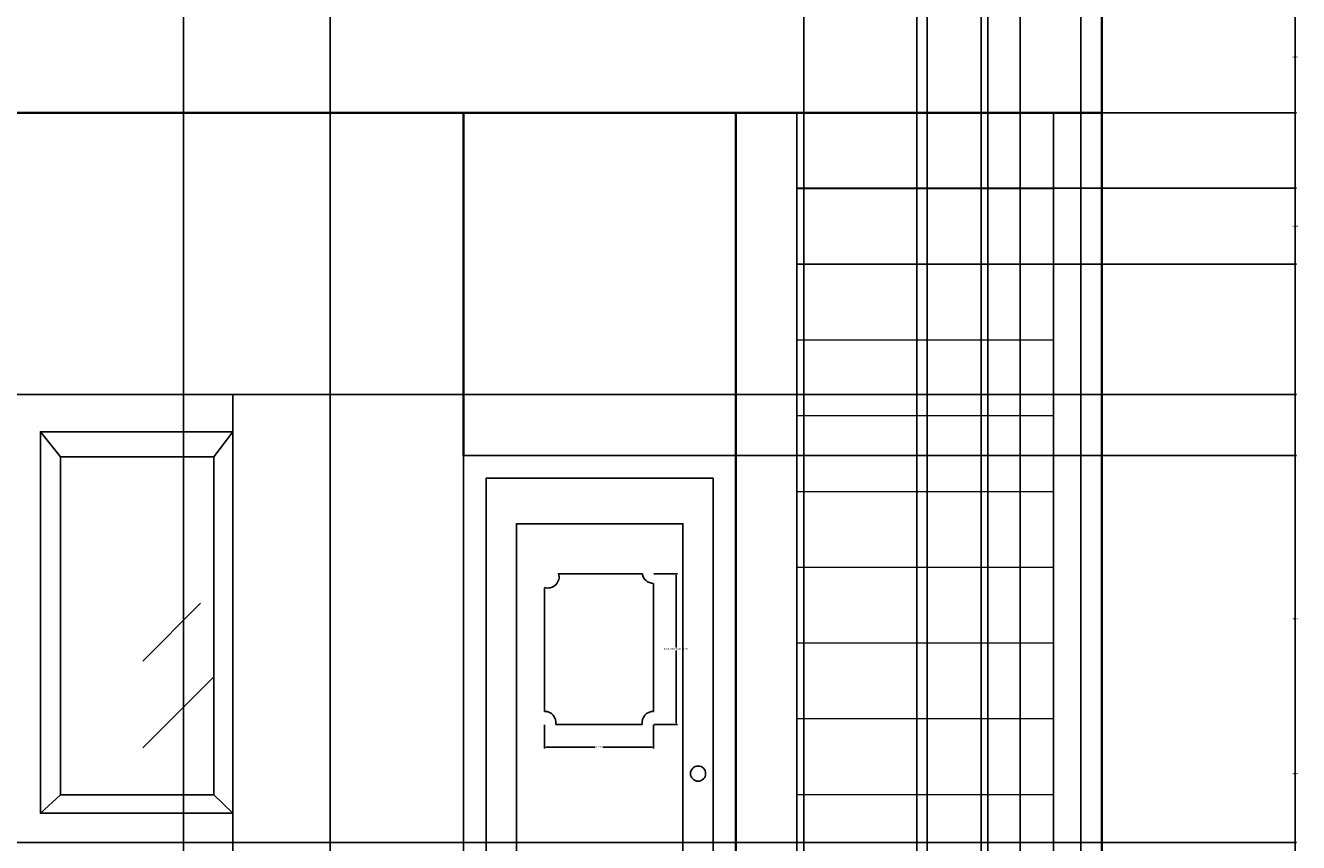
# Model space of a CAD drawing. Units: inches. Extents: x 93 to 565, y 123 to 656.
# Tile 4 of 18: x 397 to 565, y 217 to 324. Entities that reach past the tile are written whole.
import ezdxf

# ---------------------------------------------------------------- set-up
doc = ezdxf.new("R2010")
doc.units = ezdxf.units.IN
doc.header["$MEASUREMENT"] = 0
for name, color, linetype, lineweight in [('A-ANNO-DIMS', 2, 'Continuous', 18), ('A-DOOR', 3, 'Continuous', 25), ('A-ELEV', 7, 'Continuous', 35), ('A-FLOR-STRS', 6, 'Continuous', 18), ('A-GLAZ', 4, 'Continuous', 25)]:
    doc.layers.add(name, color=color, linetype=linetype, lineweight=lineweight)
doc.styles.get("Standard").update_dxf_attribs({"font": 'arial.ttf'})
doc.dimstyles.get("Standard").update_dxf_attribs({"dimtxt": 0.18, "dimasz": 0.18, "dimexe": 0.18, "dimexo": 0.0625, "dimgap": 0.09, "dimtad": 0, "dimtih": 1, "dimtoh": 1, "dimdec": 4, "dimzin": 0, "dimdsep": 46, "dimtxsty": 'Standard', "dimcen": 0.09, "dimadec": 0, "dimazin": 0, "dimtfac": 1, "dimtdec": 4, "dimtofl": 0, "dimtmove": 0, "dimatfit": 3, "dimfxl": 1, "dimtolj": 1, "dimtzin": 0, "dimarcsym": 0})

# ---------------------------------------------------------------- blocks, each defined once
blk = doc.blocks.new('*U4')
blk.add_lwpolyline([(3.12, 0.01), (0.12, 0.01), (0.12, 84.01), (36.12, 84.01), (36.12, 0.01), (33.12, 0.01)])
for points in [[(33.12, 80.99), (33.12, 0.01), (3.12, 0.01), (3.12, 80.99)], [(29.12, 6.01), (29.12, 74.99), (7.12, 74.99), (7.12, 6.01)]]:
    blk.add_lwpolyline(points, close=True)
blk.add_circle((31.12, 42.01), 1)
blk = doc.blocks.new('DOOR-PANEL-UPPER')
for points in [[(1.85, 19.9), (12.89, 19.9)], [(14.37, 18.62), (14.37, 1.72)], [(0, 1.72), (0, 18.05)], [(12.89, 0), (1.48, 0)]]:
    blk.add_lwpolyline(points)
for centre, start, end in [((0.41, 19.5), 254.1895, 15.8285), ((14.37, 20.12), 188.4141, 270), ((0, 0.22), 351.5859, 90), ((14.37, 0.22), 90, 188.4141)]:
    blk.add_arc(centre, 1.5, start, end)
blk = doc.blocks.new('WIN-CASEMENT-LARGE')
blk.add_lwpolyline([(2.67, 44.6), (0, 47.91), (25.42, 47.91), (22.89, 44.6)])
blk.add_lwpolyline([(2.67, 44.6), (22.89, 44.6), (22.89, 0), (2.67, 0)], close=True)
blk = doc.blocks.new('*D22')
at = {"layer": 'A-ANNO-DIMS', "color": 0, "lineweight": -2, "transparency": 16777216}
for p, q in [((479.94, 252.12), (483.04, 252.12)), ((482.86, 251.94), (482.86, 242.36)), ((482.86, 232.4), (482.86, 241.99)), ((479.94, 232.22), (483.04, 232.22))]:
    blk.add_line(p, q, dxfattribs=at)
at = {"layer": 'A-ANNO-DIMS', "color": 0, "transparency": 16777216}
for points in [[(482.83, 251.94), (482.89, 251.94), (482.86, 252.12)], [(482.83, 232.4), (482.89, 232.4), (482.86, 232.22)]]:
    blk.add_solid(points, dxfattribs=at)
at = {"layer": 'Defpoints', "color": 0, "transparency": 16777216}
for p in [(479.88, 252.12), (482.86, 252.12), (479.88, 232.22)]:
    blk.add_point(p, dxfattribs=at)
at = {"layer": 'A-ANNO-DIMS', "color": 0, "transparency": 16777216, "insert": (482.86, 242.17), "char_height": 0.18, "attachment_point": 5}
blk.add_mtext('\\A1;DOOR UPPER PANEL 20 TYP.', dxfattribs=at)
blk = doc.blocks.new('*D23')
at = {"layer": 'A-ANNO-DIMS', "color": 0, "lineweight": -2, "transparency": 16777216}
for p, q in [((465.5, 232.16), (465.5, 229.05)), ((479.88, 232.16), (479.88, 229.05)), ((465.68, 229.23), (472.17, 229.23)), ((479.7, 229.23), (473.21, 229.23))]:
    blk.add_line(p, q, dxfattribs=at)
at = {"layer": 'A-ANNO-DIMS', "color": 0, "transparency": 16777216}
for points in [[(465.68, 229.26), (465.68, 229.2), (465.5, 229.23)], [(479.7, 229.26), (479.7, 229.2), (479.88, 229.23)]]:
    blk.add_solid(points, dxfattribs=at)
at = {"layer": 'Defpoints', "color": 0, "transparency": 16777216}
for p in [(465.5, 232.22), (479.88, 232.22), (479.88, 229.23)]:
    blk.add_point(p, dxfattribs=at)
at = {"layer": 'A-ANNO-DIMS', "color": 0, "transparency": 16777216, "insert": (472.69, 229.23), "char_height": 0.18, "attachment_point": 5}
blk.add_mtext('\\A1;14 TYP.', dxfattribs=at)
blk = doc.blocks.new('*D29')
at = {"layer": 'A-ANNO-DIMS', "color": 0, "lineweight": -2, "transparency": 16777216}
for p, q in [((437.19, 594.34), (437.19, 134)), ((295.69, 183.67), (295.69, 134)), ((295.87, 134.18), (366.05, 134.18)), ((437.01, 134.18), (366.82, 134.18))]:
    blk.add_line(p, q, dxfattribs=at)
at = {"layer": 'A-ANNO-DIMS', "color": 0, "transparency": 16777216}
for points in [[(295.87, 134.21), (295.87, 134.15), (295.69, 134.18)], [(437.01, 134.21), (437.01, 134.15), (437.19, 134.18)]]:
    blk.add_solid(points, dxfattribs=at)
at = {"layer": 'Defpoints', "color": 0, "transparency": 16777216}
for p in [(437.19, 594.4), (295.69, 183.73), (437.19, 134.18)]:
    blk.add_point(p, dxfattribs=at)
at = {"layer": 'A-ANNO-DIMS', "color": 0, "transparency": 16777216, "insert": (366.44, 134.18), "char_height": 0.18, "attachment_point": 5}
blk.add_mtext('\\A1;141.5', dxfattribs=at)
blk = doc.blocks.new('*D30')
at = {"layer": 'A-ANNO-DIMS', "color": 0, "lineweight": -2, "transparency": 16777216}
for p, q in [((437.19, 594.34), (437.19, 134)), ((539.08, 159.67), (539.08, 134)), ((437.37, 134.18), (487.75, 134.18)), ((538.9, 134.18), (488.52, 134.18))]:
    blk.add_line(p, q, dxfattribs=at)
at = {"layer": 'A-ANNO-DIMS', "color": 0, "transparency": 16777216}
for points in [[(437.37, 134.21), (437.37, 134.15), (437.19, 134.18)], [(538.9, 134.21), (538.9, 134.15), (539.08, 134.18)]]:
    blk.add_solid(points, dxfattribs=at)
at = {"layer": 'Defpoints', "color": 0, "transparency": 16777216}
for p in [(437.19, 594.4), (539.08, 159.73), (539.08, 134.18)]:
    blk.add_point(p, dxfattribs=at)
at = {"layer": 'A-ANNO-DIMS', "color": 0, "transparency": 16777216, "insert": (488.13, 134.18), "char_height": 0.18, "attachment_point": 5}
blk.add_mtext('\\A1;101.9', dxfattribs=at)
blk = doc.blocks.new('*D31')
at = {"layer": 'A-ANNO-DIMS', "color": 0, "lineweight": -2, "transparency": 16777216}
for p, q in [((417.87, 630.4), (564.81, 630.4)), ((564.63, 630.22), (564.63, 395.25)), ((564.63, 159.91), (564.63, 394.89)), ((119.14, 159.73), (564.81, 159.73))]:
    blk.add_line(p, q, dxfattribs=at)
at = {"layer": 'A-ANNO-DIMS', "color": 0, "transparency": 16777216}
for points in [[(564.6, 630.22), (564.66, 630.22), (564.63, 630.4)], [(564.6, 159.91), (564.66, 159.91), (564.63, 159.73)]]:
    blk.add_solid(points, dxfattribs=at)
at = {"layer": 'Defpoints', "color": 0, "transparency": 16777216}
for p in [(417.81, 630.4), (564.63, 630.4), (119.08, 159.73)]:
    blk.add_point(p, dxfattribs=at)
at = {"layer": 'A-ANNO-DIMS', "color": 0, "transparency": 16777216, "insert": (564.63, 395.07), "char_height": 0.18, "attachment_point": 5}
blk.add_mtext('\\A1;470.7', dxfattribs=at)
blk = doc.blocks.new('*D37')
at = {"layer": 'A-ANNO-DIMS', "color": 0, "lineweight": -2, "transparency": 16777216}
for p, q in [((539.14, 327.73), (564.81, 327.73)), ((564.63, 327.55), (564.63, 320.52)), ((564.63, 313.13), (564.63, 320.16)), ((539.14, 312.95), (564.81, 312.95))]:
    blk.add_line(p, q, dxfattribs=at)
at = {"layer": 'A-ANNO-DIMS', "color": 0, "transparency": 16777216}
for points in [[(564.6, 327.55), (564.66, 327.55), (564.63, 327.73)], [(564.6, 313.13), (564.66, 313.13), (564.63, 312.95)]]:
    blk.add_solid(points, dxfattribs=at)
at = {"layer": 'Defpoints', "color": 0, "transparency": 16777216}
for p in [(539.08, 327.73), (564.63, 327.73), (539.08, 312.95)]:
    blk.add_point(p, dxfattribs=at)
at = {"layer": 'A-ANNO-DIMS', "color": 0, "transparency": 16777216, "insert": (564.63, 320.34), "char_height": 0.18, "attachment_point": 5}
blk.add_mtext('\\A1;14.783', dxfattribs=at)
blk = doc.blocks.new('*D56')
at = {"layer": 'A-ANNO-DIMS', "color": 0, "lineweight": -2, "transparency": 16777216}
for p, q in [((309.74, 275.71), (309.74, 134)), ((424.3, 275.71), (424.3, 134)), ((309.92, 134.18), (366.57, 134.18)), ((424.12, 134.18), (367.48, 134.18))]:
    blk.add_line(p, q, dxfattribs=at)
at = {"layer": 'A-ANNO-DIMS', "color": 0, "transparency": 16777216}
for points in [[(309.92, 134.21), (309.92, 134.15), (309.74, 134.18)], [(424.12, 134.21), (424.12, 134.15), (424.3, 134.18)]]:
    blk.add_solid(points, dxfattribs=at)
at = {"layer": 'Defpoints', "color": 0, "transparency": 16777216}
for p in [(309.74, 275.77), (424.3, 275.77), (424.3, 134.18)]:
    blk.add_point(p, dxfattribs=at)
at = {"layer": 'A-ANNO-DIMS', "color": 0, "transparency": 16777216, "insert": (367.02, 134.18), "char_height": 0.18, "attachment_point": 5}
blk.add_mtext('\\A1;114.56', dxfattribs=at)
blk = doc.blocks.new('*D57')
at = {"layer": 'A-ANNO-DIMS', "color": 0, "lineweight": -2, "transparency": 16777216}
for p, q in [((424.37, 275.77), (564.81, 275.77)), ((564.63, 275.59), (564.63, 246.38)), ((564.63, 216.81), (564.63, 246.02)), ((424.37, 216.63), (564.81, 216.63))]:
    blk.add_line(p, q, dxfattribs=at)
at = {"layer": 'A-ANNO-DIMS', "color": 0, "transparency": 16777216}
for points in [[(564.6, 275.59), (564.66, 275.59), (564.63, 275.77)], [(564.6, 216.81), (564.66, 216.81), (564.63, 216.63)]]:
    blk.add_solid(points, dxfattribs=at)
at = {"layer": 'Defpoints', "color": 0, "transparency": 16777216}
for p in [(424.3, 275.77), (564.63, 275.77), (424.3, 216.63)]:
    blk.add_point(p, dxfattribs=at)
at = {"layer": 'A-ANNO-DIMS', "color": 0, "transparency": 16777216, "insert": (564.63, 246.2), "char_height": 0.18, "attachment_point": 5}
blk.add_mtext('\\A1;59.14', dxfattribs=at)
blk = doc.blocks.new('*D59')
at = {"layer": 'A-ANNO-DIMS', "color": 0, "lineweight": -2, "transparency": 16777216}
for p, q in [((454.77, 267.67), (454.77, 134)), ((490.77, 267.67), (490.77, 134)), ((454.95, 134.18), (472.55, 134.18)), ((490.59, 134.18), (472.99, 134.18))]:
    blk.add_line(p, q, dxfattribs=at)
at = {"layer": 'A-ANNO-DIMS', "color": 0, "transparency": 16777216}
for points in [[(454.95, 134.21), (454.95, 134.15), (454.77, 134.18)], [(490.59, 134.21), (490.59, 134.15), (490.77, 134.18)]]:
    blk.add_solid(points, dxfattribs=at)
at = {"layer": 'Defpoints', "color": 0, "transparency": 16777216}
for p in [(454.77, 267.73), (490.77, 267.73), (490.77, 134.18)]:
    blk.add_point(p, dxfattribs=at)
at = {"layer": 'A-ANNO-DIMS', "color": 0, "transparency": 16777216, "insert": (472.77, 134.18), "char_height": 0.18, "attachment_point": 5}
blk.add_mtext('\\A1;36', dxfattribs=at)
blk = doc.blocks.new('*D60')
at = {"layer": 'A-ANNO-DIMS', "color": 0, "lineweight": -2, "transparency": 16777216}
for p, q in [((490.83, 267.73), (564.81, 267.73)), ((564.63, 267.55), (564.63, 225.91)), ((564.63, 183.91), (564.63, 225.55)), ((490.83, 183.73), (564.81, 183.73))]:
    blk.add_line(p, q, dxfattribs=at)
at = {"layer": 'A-ANNO-DIMS', "color": 0, "transparency": 16777216}
for points in [[(564.6, 267.55), (564.66, 267.55), (564.63, 267.73)], [(564.6, 183.91), (564.66, 183.91), (564.63, 183.73)]]:
    blk.add_solid(points, dxfattribs=at)
at = {"layer": 'Defpoints', "color": 0, "transparency": 16777216}
for p in [(490.77, 267.73), (564.63, 267.73), (490.77, 183.73)]:
    blk.add_point(p, dxfattribs=at)
at = {"layer": 'A-ANNO-DIMS', "color": 0, "transparency": 16777216, "insert": (564.63, 225.73), "char_height": 0.18, "attachment_point": 5}
blk.add_mtext('\\A1;84', dxfattribs=at)
blk = doc.blocks.new('*D62')
at = {"layer": 'A-ANNO-DIMS', "color": 0, "lineweight": -2, "transparency": 16777216}
for p, q in [((498.79, 312.92), (498.79, 134)), ((532.69, 312.92), (532.69, 134)), ((498.97, 134.18), (515.42, 134.18)), ((532.51, 134.18), (516.07, 134.18))]:
    blk.add_line(p, q, dxfattribs=at)
at = {"layer": 'A-ANNO-DIMS', "color": 0, "transparency": 16777216}
for points in [[(498.97, 134.21), (498.97, 134.15), (498.79, 134.18)], [(532.51, 134.21), (532.51, 134.15), (532.69, 134.18)]]:
    blk.add_solid(points, dxfattribs=at)
at = {"layer": 'Defpoints', "color": 0, "transparency": 16777216}
for p in [(498.79, 312.99), (532.69, 312.99), (532.69, 134.18)]:
    blk.add_point(p, dxfattribs=at)
at = {"layer": 'A-ANNO-DIMS', "color": 0, "transparency": 16777216, "insert": (515.74, 134.18), "char_height": 0.18, "attachment_point": 5}
blk.add_mtext('\\A1;33.9', dxfattribs=at)
blk = doc.blocks.new('*D63')
at = {"layer": 'A-ANNO-DIMS', "color": 0, "lineweight": -2, "transparency": 16777216}
for p, q in [((498.86, 302.99), (564.81, 302.99)), ((564.63, 302.81), (564.63, 298.17)), ((564.63, 293.17), (564.63, 297.8)), ((498.86, 292.99), (564.81, 292.99))]:
    blk.add_line(p, q, dxfattribs=at)
at = {"layer": 'A-ANNO-DIMS', "color": 0, "transparency": 16777216}
for points in [[(564.6, 302.81), (564.66, 302.81), (564.63, 302.99)], [(564.6, 293.17), (564.66, 293.17), (564.63, 292.99)]]:
    blk.add_solid(points, dxfattribs=at)
at = {"layer": 'Defpoints', "color": 0, "transparency": 16777216}
for p in [(498.79, 302.99), (498.79, 292.99), (564.63, 292.99)]:
    blk.add_point(p, dxfattribs=at)
at = {"layer": 'A-ANNO-DIMS', "color": 0, "transparency": 16777216, "insert": (564.63, 297.99), "char_height": 0.18, "attachment_point": 5}
blk.add_mtext('\\A1;10', dxfattribs=at)
blk = doc.blocks.new('*D90')
at = {"layer": 'A-ANNO-DIMS', "color": 0, "lineweight": -2, "transparency": 16777216}
for p, q in [((417.81, 594.34), (417.81, 134)), ((437.19, 594.34), (437.19, 134)), ((417.99, 134.18), (427.11, 134.18)), ((437.01, 134.18), (427.88, 134.18))]:
    blk.add_line(p, q, dxfattribs=at)
at = {"layer": 'A-ANNO-DIMS', "color": 0, "transparency": 16777216}
for points in [[(417.99, 134.21), (417.99, 134.15), (417.81, 134.18)], [(437.01, 134.21), (437.01, 134.15), (437.19, 134.18)]]:
    blk.add_solid(points, dxfattribs=at)
at = {"layer": 'Defpoints', "color": 0, "transparency": 16777216}
for p in [(417.81, 594.4), (437.19, 594.4), (437.19, 134.18)]:
    blk.add_point(p, dxfattribs=at)
at = {"layer": 'A-ANNO-DIMS', "color": 0, "transparency": 16777216, "insert": (427.5, 134.18), "char_height": 0.18, "attachment_point": 5}
blk.add_mtext('\\A1;19.38', dxfattribs=at)
blk = doc.blocks.new('*D91')
at = {"layer": 'A-ANNO-DIMS', "color": 0, "lineweight": -2, "transparency": 16777216}
for p, q in [((499.73, 599.75), (499.73, 134)), ((437.19, 594.34), (437.19, 134)), ((437.37, 134.18), (468.07, 134.18)), ((499.55, 134.18), (468.85, 134.18))]:
    blk.add_line(p, q, dxfattribs=at)
at = {"layer": 'A-ANNO-DIMS', "color": 0, "transparency": 16777216}
for points in [[(437.37, 134.21), (437.37, 134.15), (437.19, 134.18)], [(499.55, 134.21), (499.55, 134.15), (499.73, 134.18)]]:
    blk.add_solid(points, dxfattribs=at)
at = {"layer": 'Defpoints', "color": 0, "transparency": 16777216}
for p in [(499.73, 599.82), (437.19, 594.4), (499.73, 134.18)]:
    blk.add_point(p, dxfattribs=at)
at = {"layer": 'A-ANNO-DIMS', "color": 0, "transparency": 16777216, "insert": (468.46, 134.18), "char_height": 0.18, "attachment_point": 5}
blk.add_mtext('\\A1;62.54', dxfattribs=at)
blk = doc.blocks.new('*D92')
at = {"layer": 'A-ANNO-DIMS', "color": 0, "lineweight": -2, "transparency": 16777216}
for p, q in [((523.14, 603.14), (523.14, 134)), ((499.73, 599.75), (499.73, 134)), ((499.91, 134.18), (510.97, 134.18)), ((522.96, 134.18), (511.9, 134.18))]:
    blk.add_line(p, q, dxfattribs=at)
at = {"layer": 'A-ANNO-DIMS', "color": 0, "transparency": 16777216}
for points in [[(499.91, 134.21), (499.91, 134.15), (499.73, 134.18)], [(522.96, 134.21), (522.96, 134.15), (523.14, 134.18)]]:
    blk.add_solid(points, dxfattribs=at)
at = {"layer": 'Defpoints', "color": 0, "transparency": 16777216}
for p in [(523.14, 603.2), (499.73, 599.82), (523.14, 134.18)]:
    blk.add_point(p, dxfattribs=at)
at = {"layer": 'A-ANNO-DIMS', "color": 0, "transparency": 16777216, "insert": (511.44, 134.18), "char_height": 0.18, "attachment_point": 5}
blk.add_mtext('\\A1;23.412', dxfattribs=at)
blk = doc.blocks.new('*D93')
at = {"layer": 'A-ANNO-DIMS', "color": 0, "lineweight": -2, "transparency": 16777216}
for p, q in [((523.14, 603.14), (523.14, 134)), ((539.08, 594.34), (539.08, 134)), ((523.32, 134.18), (530.66, 134.18)), ((538.9, 134.18), (531.57, 134.18))]:
    blk.add_line(p, q, dxfattribs=at)
at = {"layer": 'A-ANNO-DIMS', "color": 0, "transparency": 16777216}
for points in [[(523.32, 134.21), (523.32, 134.15), (523.14, 134.18)], [(538.9, 134.21), (538.9, 134.15), (539.08, 134.18)]]:
    blk.add_solid(points, dxfattribs=at)
at = {"layer": 'Defpoints', "color": 0, "transparency": 16777216}
for p in [(523.14, 603.2), (539.08, 594.4), (539.08, 134.18)]:
    blk.add_point(p, dxfattribs=at)
at = {"layer": 'A-ANNO-DIMS', "color": 0, "transparency": 16777216, "insert": (531.11, 134.18), "char_height": 0.18, "attachment_point": 5}
blk.add_mtext('\\A1;15.938', dxfattribs=at)
blk = doc.blocks.new('*D108')
at = {"layer": 'A-ANNO-DIMS', "color": 0, "lineweight": -2, "transparency": 16777216}
for p, q in [((437.19, 594.34), (437.19, 134)), ((295.69, 183.67), (295.69, 134)), ((295.87, 134.18), (365.93, 134.18)), ((437.01, 134.18), (366.95, 134.18))]:
    blk.add_line(p, q, dxfattribs=at)
at = {"layer": 'A-ANNO-DIMS', "color": 0, "transparency": 16777216}
for points in [[(295.87, 134.21), (295.87, 134.15), (295.69, 134.18)], [(437.01, 134.21), (437.01, 134.15), (437.19, 134.18)]]:
    blk.add_solid(points, dxfattribs=at)
at = {"layer": 'Defpoints', "color": 0, "transparency": 16777216}
for p in [(437.19, 594.4), (295.69, 183.73), (437.19, 134.18)]:
    blk.add_point(p, dxfattribs=at)
at = {"layer": 'A-ANNO-DIMS', "color": 0, "transparency": 16777216, "insert": (366.44, 134.18), "char_height": 0.18, "attachment_point": 5}
blk.add_mtext('\\A1;141.501', dxfattribs=at)
blk = doc.blocks.new('*D109')
at = {"layer": 'A-ANNO-DIMS', "color": 0, "lineweight": -2, "transparency": 16777216}
for p, q in [((437.19, 594.34), (437.19, 134)), ((539.08, 159.67), (539.08, 134)), ((437.37, 134.18), (487.63, 134.18)), ((538.9, 134.18), (488.64, 134.18))]:
    blk.add_line(p, q, dxfattribs=at)
at = {"layer": 'A-ANNO-DIMS', "color": 0, "transparency": 16777216}
for points in [[(437.37, 134.21), (437.37, 134.15), (437.19, 134.18)], [(538.9, 134.21), (538.9, 134.15), (539.08, 134.18)]]:
    blk.add_solid(points, dxfattribs=at)
at = {"layer": 'Defpoints', "color": 0, "transparency": 16777216}
for p in [(437.19, 594.4), (539.08, 159.73), (539.08, 134.18)]:
    blk.add_point(p, dxfattribs=at)
at = {"layer": 'A-ANNO-DIMS', "color": 0, "transparency": 16777216, "insert": (488.13, 134.18), "char_height": 0.18, "attachment_point": 5}
blk.add_mtext('\\A1;101.891', dxfattribs=at)
blk = doc.blocks.new('*D110')
at = {"layer": 'A-ANNO-DIMS', "color": 0, "lineweight": -2, "transparency": 16777216}
for p, q in [((417.87, 630.4), (564.81, 630.4)), ((564.63, 630.22), (564.63, 395.25)), ((564.63, 159.91), (564.63, 394.89)), ((119.14, 159.73), (564.81, 159.73))]:
    blk.add_line(p, q, dxfattribs=at)
at = {"layer": 'A-ANNO-DIMS', "color": 0, "transparency": 16777216}
for points in [[(564.6, 630.22), (564.66, 630.22), (564.63, 630.4)], [(564.6, 159.91), (564.66, 159.91), (564.63, 159.73)]]:
    blk.add_solid(points, dxfattribs=at)
at = {"layer": 'Defpoints', "color": 0, "transparency": 16777216}
for p in [(417.81, 630.4), (564.63, 630.4), (119.08, 159.73)]:
    blk.add_point(p, dxfattribs=at)
at = {"layer": 'A-ANNO-DIMS', "color": 0, "transparency": 16777216, "insert": (564.63, 395.07), "char_height": 0.18, "attachment_point": 5}
blk.add_mtext('\\A1;470.673', dxfattribs=at)
blk = doc.blocks.new('*D116')
at = {"layer": 'A-ANNO-DIMS', "color": 0, "lineweight": -2, "transparency": 16777216}
for p, q in [((539.14, 327.73), (564.81, 327.73)), ((564.63, 327.55), (564.63, 320.52)), ((564.63, 313.13), (564.63, 320.16)), ((539.14, 312.95), (564.81, 312.95))]:
    blk.add_line(p, q, dxfattribs=at)
at = {"layer": 'A-ANNO-DIMS', "color": 0, "transparency": 16777216}
for points in [[(564.6, 327.55), (564.66, 327.55), (564.63, 327.73)], [(564.6, 313.13), (564.66, 313.13), (564.63, 312.95)]]:
    blk.add_solid(points, dxfattribs=at)
at = {"layer": 'Defpoints', "color": 0, "transparency": 16777216}
for p in [(539.08, 327.73), (564.63, 327.73), (539.08, 312.95)]:
    blk.add_point(p, dxfattribs=at)
at = {"layer": 'A-ANNO-DIMS', "color": 0, "transparency": 16777216, "insert": (564.63, 320.34), "char_height": 0.18, "attachment_point": 5}
blk.add_mtext('\\A1;14.783', dxfattribs=at)
blk = doc.blocks.new('*D135')
at = {"layer": 'A-ANNO-DIMS', "color": 0, "lineweight": -2, "transparency": 16777216}
for p, q in [((309.74, 275.71), (309.74, 134)), ((424.3, 275.71), (424.3, 134)), ((309.92, 134.18), (366.5, 134.18)), ((424.12, 134.18), (367.55, 134.18))]:
    blk.add_line(p, q, dxfattribs=at)
at = {"layer": 'A-ANNO-DIMS', "color": 0, "transparency": 16777216}
for points in [[(309.92, 134.21), (309.92, 134.15), (309.74, 134.18)], [(424.12, 134.21), (424.12, 134.15), (424.3, 134.18)]]:
    blk.add_solid(points, dxfattribs=at)
at = {"layer": 'Defpoints', "color": 0, "transparency": 16777216}
for p in [(309.74, 275.77), (424.3, 275.77), (424.3, 134.18)]:
    blk.add_point(p, dxfattribs=at)
at = {"layer": 'A-ANNO-DIMS', "color": 0, "transparency": 16777216, "insert": (367.02, 134.18), "char_height": 0.18, "attachment_point": 5}
blk.add_mtext('\\A1;114.560', dxfattribs=at)
blk = doc.blocks.new('*D136')
at = {"layer": 'A-ANNO-DIMS', "color": 0, "lineweight": -2, "transparency": 16777216}
for p, q in [((424.37, 275.77), (564.81, 275.77)), ((564.63, 275.59), (564.63, 246.38)), ((564.63, 216.81), (564.63, 246.02)), ((424.37, 216.63), (564.81, 216.63))]:
    blk.add_line(p, q, dxfattribs=at)
at = {"layer": 'A-ANNO-DIMS', "color": 0, "transparency": 16777216}
for points in [[(564.6, 275.59), (564.66, 275.59), (564.63, 275.77)], [(564.6, 216.81), (564.66, 216.81), (564.63, 216.63)]]:
    blk.add_solid(points, dxfattribs=at)
at = {"layer": 'Defpoints', "color": 0, "transparency": 16777216}
for p in [(424.3, 275.77), (564.63, 275.77), (424.3, 216.63)]:
    blk.add_point(p, dxfattribs=at)
at = {"layer": 'A-ANNO-DIMS', "color": 0, "transparency": 16777216, "insert": (564.63, 246.2), "char_height": 0.18, "attachment_point": 5}
blk.add_mtext('\\A1;59.144', dxfattribs=at)
blk = doc.blocks.new('*D138')
at = {"layer": 'A-ANNO-DIMS', "color": 0, "lineweight": -2, "transparency": 16777216}
for p, q in [((454.77, 267.67), (454.77, 134)), ((490.77, 267.67), (490.77, 134)), ((454.95, 134.18), (472.31, 134.18)), ((490.59, 134.18), (473.23, 134.18))]:
    blk.add_line(p, q, dxfattribs=at)
at = {"layer": 'A-ANNO-DIMS', "color": 0, "transparency": 16777216}
for points in [[(454.95, 134.21), (454.95, 134.15), (454.77, 134.18)], [(490.59, 134.21), (490.59, 134.15), (490.77, 134.18)]]:
    blk.add_solid(points, dxfattribs=at)
at = {"layer": 'Defpoints', "color": 0, "transparency": 16777216}
for p in [(454.77, 267.73), (490.77, 267.73), (490.77, 134.18)]:
    blk.add_point(p, dxfattribs=at)
at = {"layer": 'A-ANNO-DIMS', "color": 0, "transparency": 16777216, "insert": (472.77, 134.18), "char_height": 0.18, "attachment_point": 5}
blk.add_mtext('\\A1;36.000', dxfattribs=at)
blk = doc.blocks.new('*D139')
at = {"layer": 'A-ANNO-DIMS', "color": 0, "lineweight": -2, "transparency": 16777216}
for p, q in [((490.83, 267.73), (564.81, 267.73)), ((564.63, 267.55), (564.63, 225.91)), ((564.63, 183.91), (564.63, 225.55)), ((490.83, 183.73), (564.81, 183.73))]:
    blk.add_line(p, q, dxfattribs=at)
at = {"layer": 'A-ANNO-DIMS', "color": 0, "transparency": 16777216}
for points in [[(564.6, 267.55), (564.66, 267.55), (564.63, 267.73)], [(564.6, 183.91), (564.66, 183.91), (564.63, 183.73)]]:
    blk.add_solid(points, dxfattribs=at)
at = {"layer": 'Defpoints', "color": 0, "transparency": 16777216}
for p in [(490.77, 267.73), (564.63, 267.73), (490.77, 183.73)]:
    blk.add_point(p, dxfattribs=at)
at = {"layer": 'A-ANNO-DIMS', "color": 0, "transparency": 16777216, "insert": (564.63, 225.73), "char_height": 0.18, "attachment_point": 5}
blk.add_mtext('\\A1;84.000', dxfattribs=at)
blk = doc.blocks.new('*D141')
at = {"layer": 'A-ANNO-DIMS', "color": 0, "lineweight": -2, "transparency": 16777216}
for p, q in [((498.79, 312.92), (498.79, 134)), ((532.69, 312.92), (532.69, 134)), ((498.97, 134.18), (515.28, 134.18)), ((532.51, 134.18), (516.21, 134.18))]:
    blk.add_line(p, q, dxfattribs=at)
at = {"layer": 'A-ANNO-DIMS', "color": 0, "transparency": 16777216}
for points in [[(498.97, 134.21), (498.97, 134.15), (498.79, 134.18)], [(532.51, 134.21), (532.51, 134.15), (532.69, 134.18)]]:
    blk.add_solid(points, dxfattribs=at)
at = {"layer": 'Defpoints', "color": 0, "transparency": 16777216}
for p in [(498.79, 312.99), (532.69, 312.99), (532.69, 134.18)]:
    blk.add_point(p, dxfattribs=at)
at = {"layer": 'A-ANNO-DIMS', "color": 0, "transparency": 16777216, "insert": (515.74, 134.18), "char_height": 0.18, "attachment_point": 5}
blk.add_mtext('\\A1;33.897', dxfattribs=at)
blk = doc.blocks.new('*D142')
at = {"layer": 'A-ANNO-DIMS', "color": 0, "lineweight": -2, "transparency": 16777216}
for p, q in [((498.86, 302.99), (564.81, 302.99)), ((564.63, 302.81), (564.63, 298.17)), ((564.63, 293.17), (564.63, 297.8)), ((498.86, 292.99), (564.81, 292.99))]:
    blk.add_line(p, q, dxfattribs=at)
at = {"layer": 'A-ANNO-DIMS', "color": 0, "transparency": 16777216}
for points in [[(564.6, 302.81), (564.66, 302.81), (564.63, 302.99)], [(564.6, 293.17), (564.66, 293.17), (564.63, 292.99)]]:
    blk.add_solid(points, dxfattribs=at)
at = {"layer": 'Defpoints', "color": 0, "transparency": 16777216}
for p in [(498.79, 302.99), (498.79, 292.99), (564.63, 292.99)]:
    blk.add_point(p, dxfattribs=at)
at = {"layer": 'A-ANNO-DIMS', "color": 0, "transparency": 16777216, "insert": (564.63, 297.99), "char_height": 0.18, "attachment_point": 5}
blk.add_mtext('\\A1;10.000', dxfattribs=at)
blk = doc.blocks.new('*D169')
at = {"layer": 'A-ANNO-DIMS', "color": 0, "lineweight": -2, "transparency": 16777216}
for p, q in [((417.81, 594.34), (417.81, 134)), ((437.19, 594.34), (437.19, 134)), ((417.99, 134.18), (427.04, 134.18)), ((437.01, 134.18), (427.95, 134.18))]:
    blk.add_line(p, q, dxfattribs=at)
at = {"layer": 'A-ANNO-DIMS', "color": 0, "transparency": 16777216}
for points in [[(417.99, 134.21), (417.99, 134.15), (417.81, 134.18)], [(437.01, 134.21), (437.01, 134.15), (437.19, 134.18)]]:
    blk.add_solid(points, dxfattribs=at)
at = {"layer": 'Defpoints', "color": 0, "transparency": 16777216}
for p in [(417.81, 594.4), (437.19, 594.4), (437.19, 134.18)]:
    blk.add_point(p, dxfattribs=at)
at = {"layer": 'A-ANNO-DIMS', "color": 0, "transparency": 16777216, "insert": (427.5, 134.18), "char_height": 0.18, "attachment_point": 5}
blk.add_mtext('\\A1;19.379', dxfattribs=at)
blk = doc.blocks.new('*D170')
at = {"layer": 'A-ANNO-DIMS', "color": 0, "lineweight": -2, "transparency": 16777216}
for p, q in [((499.73, 599.75), (499.73, 134)), ((437.19, 594.34), (437.19, 134)), ((437.37, 134.18), (468.01, 134.18)), ((499.55, 134.18), (468.91, 134.18))]:
    blk.add_line(p, q, dxfattribs=at)
at = {"layer": 'A-ANNO-DIMS', "color": 0, "transparency": 16777216}
for points in [[(437.37, 134.21), (437.37, 134.15), (437.19, 134.18)], [(499.55, 134.21), (499.55, 134.15), (499.73, 134.18)]]:
    blk.add_solid(points, dxfattribs=at)
at = {"layer": 'Defpoints', "color": 0, "transparency": 16777216}
for p in [(499.73, 599.82), (437.19, 594.4), (499.73, 134.18)]:
    blk.add_point(p, dxfattribs=at)
at = {"layer": 'A-ANNO-DIMS', "color": 0, "transparency": 16777216, "insert": (468.46, 134.18), "char_height": 0.18, "attachment_point": 5}
blk.add_mtext('\\A1;62.541', dxfattribs=at)
blk = doc.blocks.new('*D171')
at = {"layer": 'A-ANNO-DIMS', "color": 0, "lineweight": -2, "transparency": 16777216}
for p, q in [((523.14, 603.14), (523.14, 134)), ((499.73, 599.75), (499.73, 134)), ((499.91, 134.18), (510.97, 134.18)), ((522.96, 134.18), (511.9, 134.18))]:
    blk.add_line(p, q, dxfattribs=at)
at = {"layer": 'A-ANNO-DIMS', "color": 0, "transparency": 16777216}
for points in [[(499.91, 134.21), (499.91, 134.15), (499.73, 134.18)], [(522.96, 134.21), (522.96, 134.15), (523.14, 134.18)]]:
    blk.add_solid(points, dxfattribs=at)
at = {"layer": 'Defpoints', "color": 0, "transparency": 16777216}
for p in [(523.14, 603.2), (499.73, 599.82), (523.14, 134.18)]:
    blk.add_point(p, dxfattribs=at)
at = {"layer": 'A-ANNO-DIMS', "color": 0, "transparency": 16777216, "insert": (511.44, 134.18), "char_height": 0.18, "attachment_point": 5}
blk.add_mtext('\\A1;23.412', dxfattribs=at)
blk = doc.blocks.new('*D172')
at = {"layer": 'A-ANNO-DIMS', "color": 0, "lineweight": -2, "transparency": 16777216}
for p, q in [((523.14, 603.14), (523.14, 134)), ((539.08, 594.34), (539.08, 134)), ((523.32, 134.18), (530.66, 134.18)), ((538.9, 134.18), (531.57, 134.18))]:
    blk.add_line(p, q, dxfattribs=at)
at = {"layer": 'A-ANNO-DIMS', "color": 0, "transparency": 16777216}
for points in [[(523.32, 134.21), (523.32, 134.15), (523.14, 134.18)], [(538.9, 134.21), (538.9, 134.15), (539.08, 134.18)]]:
    blk.add_solid(points, dxfattribs=at)
at = {"layer": 'Defpoints', "color": 0, "transparency": 16777216}
for p in [(523.14, 603.2), (539.08, 594.4), (539.08, 134.18)]:
    blk.add_point(p, dxfattribs=at)
at = {"layer": 'A-ANNO-DIMS', "color": 0, "transparency": 16777216, "insert": (531.11, 134.18), "char_height": 0.18, "attachment_point": 5}
blk.add_mtext('\\A1;15.938', dxfattribs=at)
blk = doc.blocks.new('*D180')
at = {"layer": 'A-ANNO-DIMS', "color": 0, "lineweight": -2, "transparency": 16777216}
for p, q in [((514.64, 348.49), (514.64, 134)), ((516.01, 331.37), (516.01, 134)), ((514.82, 134.18), (514.94, 134.18)), ((515.83, 134.18), (515.71, 134.18))]:
    blk.add_line(p, q, dxfattribs=at)
at = {"layer": 'A-ANNO-DIMS', "color": 0, "transparency": 16777216}
for points in [[(514.82, 134.21), (514.82, 134.15), (514.64, 134.18)], [(515.83, 134.21), (515.83, 134.15), (516.01, 134.18)]]:
    blk.add_solid(points, dxfattribs=at)
at = {"layer": 'Defpoints', "color": 0, "transparency": 16777216}
for p in [(514.64, 348.55), (516.01, 331.43), (516.01, 134.18)]:
    blk.add_point(p, dxfattribs=at)
at = {"layer": 'A-ANNO-DIMS', "color": 0, "transparency": 16777216, "insert": (515.33, 134.18), "char_height": 0.18, "attachment_point": 5}
blk.add_mtext('\\A1;1.367', dxfattribs=at)
blk = doc.blocks.new('*D181')
at = {"layer": 'A-ANNO-DIMS', "color": 0, "lineweight": -2, "transparency": 16777216}
for p, q in [((516.01, 331.37), (516.01, 134)), ((524.02, 331.37), (524.02, 134)), ((516.19, 134.18), (519.62, 134.18)), ((523.84, 134.18), (520.41, 134.18))]:
    blk.add_line(p, q, dxfattribs=at)
at = {"layer": 'A-ANNO-DIMS', "color": 0, "transparency": 16777216}
for points in [[(516.19, 134.21), (516.19, 134.15), (516.01, 134.18)], [(523.84, 134.21), (523.84, 134.15), (524.02, 134.18)]]:
    blk.add_solid(points, dxfattribs=at)
at = {"layer": 'Defpoints', "color": 0, "transparency": 16777216}
for p in [(516.01, 331.43), (524.02, 331.43), (524.02, 134.18)]:
    blk.add_point(p, dxfattribs=at)
at = {"layer": 'A-ANNO-DIMS', "color": 0, "transparency": 16777216, "insert": (520.01, 134.18), "char_height": 0.18, "attachment_point": 5}
blk.add_mtext('\\A1;8.007', dxfattribs=at)
blk = doc.blocks.new('*D182')
at = {"layer": 'A-ANNO-DIMS', "color": 0, "lineweight": -2, "transparency": 16777216}
for p, q in [((524.02, 331.37), (524.02, 134)), ((528.31, 330.19), (528.31, 134)), ((524.2, 134.18), (525.77, 134.18)), ((528.13, 134.18), (526.56, 134.18))]:
    blk.add_line(p, q, dxfattribs=at)
at = {"layer": 'A-ANNO-DIMS', "color": 0, "transparency": 16777216}
for points in [[(524.2, 134.21), (524.2, 134.15), (524.02, 134.18)], [(528.13, 134.21), (528.13, 134.15), (528.31, 134.18)]]:
    blk.add_solid(points, dxfattribs=at)
at = {"layer": 'Defpoints', "color": 0, "transparency": 16777216}
for p in [(524.02, 331.43), (528.31, 330.25), (528.31, 134.18)]:
    blk.add_point(p, dxfattribs=at)
at = {"layer": 'A-ANNO-DIMS', "color": 0, "transparency": 16777216, "insert": (526.17, 134.18), "char_height": 0.18, "attachment_point": 5}
blk.add_mtext('\\A1;4.297', dxfattribs=at)
blk = doc.blocks.new('*D183')
at = {"layer": 'A-ANNO-DIMS', "color": 0, "lineweight": -2, "transparency": 16777216}
for p, q in [((528.31, 330.19), (528.31, 134)), ((536.32, 330.19), (536.32, 134)), ((528.49, 134.18), (531.92, 134.18)), ((536.14, 134.18), (532.71, 134.18))]:
    blk.add_line(p, q, dxfattribs=at)
at = {"layer": 'A-ANNO-DIMS', "color": 0, "transparency": 16777216}
for points in [[(528.49, 134.21), (528.49, 134.15), (528.31, 134.18)], [(536.14, 134.21), (536.14, 134.15), (536.32, 134.18)]]:
    blk.add_solid(points, dxfattribs=at)
at = {"layer": 'Defpoints', "color": 0, "transparency": 16777216}
for p in [(528.31, 330.25), (536.32, 330.25), (536.32, 134.18)]:
    blk.add_point(p, dxfattribs=at)
at = {"layer": 'A-ANNO-DIMS', "color": 0, "transparency": 16777216, "insert": (532.32, 134.18), "char_height": 0.18, "attachment_point": 5}
blk.add_mtext('\\A1;8.007', dxfattribs=at)
blk = doc.blocks.new('*D184')
at = {"layer": 'A-ANNO-DIMS', "color": 0, "lineweight": -2, "transparency": 16777216}
for p, q in [((536.32, 330.19), (536.32, 134)), ((539.08, 327.67), (539.08, 134)), ((536.5, 134.18), (537.31, 134.18)), ((538.9, 134.18), (538.1, 134.18))]:
    blk.add_line(p, q, dxfattribs=at)
at = {"layer": 'A-ANNO-DIMS', "color": 0, "transparency": 16777216}
for points in [[(536.5, 134.21), (536.5, 134.15), (536.32, 134.18)], [(538.9, 134.21), (538.9, 134.15), (539.08, 134.18)]]:
    blk.add_solid(points, dxfattribs=at)
at = {"layer": 'Defpoints', "color": 0, "transparency": 16777216}
for p in [(536.32, 330.25), (539.08, 327.73), (539.08, 134.18)]:
    blk.add_point(p, dxfattribs=at)
at = {"layer": 'A-ANNO-DIMS', "color": 0, "transparency": 16777216, "insert": (537.7, 134.18), "char_height": 0.18, "attachment_point": 5}
blk.add_mtext('\\A1;2.758', dxfattribs=at)

msp = doc.modelspace()

# ---------------------------------------------------------------- hatches: boundary and pattern name
at = {"layer": 'A-GLAZ'}
h = msp.add_hatch(dxfattribs=at)
h.set_pattern_fill('GOST_GLASS', color=256, scale=5.4)
h.set_pattern_definition([(45, (0, 0), (45.8205, 0), [27, -37.8]), (45, (11.455, 0), (45.8205, 0), [10.8, -54]), (45, (0, 11.455), (45.8205, 0), [10.8, -54])])
h.paths.add_polyline_path([(236.4617, 274.9686), (216.0562, 274.9686), (216.0562, 220.3466), (236.4617, 220.3466)])
h.paths.add_polyline_path([(258.8673, 274.9686), (237.4617, 274.9686), (237.4617, 220.3466), (258.8673, 220.3466)])
h.paths.add_polyline_path([(332.6288, 267.5414), (312.4161, 267.5414), (312.4161, 222.941), (332.6288, 222.941)])
h.paths.add_polyline_path([(366.6285, 270.8489), (341.2098, 270.8489), (341.2098, 220.4891), (366.6285, 220.4891)])
h.paths.add_polyline_path([(343.8825, 222.941), (364.0951, 222.941), (364.0951, 267.5414), (343.8825, 267.5414)], flags=16)
h.paths.add_polyline_path([(392.4256, 267.5414), (372.2129, 267.5414), (372.2129, 222.941), (392.4256, 222.941)])
h.paths.add_polyline_path([(421.7937, 267.5414), (401.581, 267.5414), (401.581, 222.941), (421.7937, 222.941)])

# ---------------------------------------------------------------- linework, layer by layer
at = {"layer": 'A-ELEV'}
for p, q in [((539.0794, 183.7323), (539.0794, 327.7323)), ((286.6874, 312.9491), (539.0794, 312.9491)), ((454.7699, 267.7323), (454.7699, 312.9491)), ((490.7699, 312.9491), (490.7699, 183.7323))]:
    msp.add_line(p, q, dxfattribs=at)
at = {"layer": 'A-FLOR-STRS'}
for p, q in [((498.7947, 312.985), (532.6916, 312.985)), ((498.7947, 312.985), (498.7947, 183.7323)), ((532.6916, 312.985), (532.6916, 183.7323)), ((498.7947, 302.985), (532.6916, 302.985)), ((498.7947, 292.985), (532.6916, 292.985)), ((498.7947, 282.985), (532.6916, 282.985)), ((498.7947, 272.985), (532.6916, 272.985)), ((498.7947, 262.985), (532.6916, 262.985)), ((498.7947, 252.985), (532.6916, 252.985)), ((498.7947, 242.985), (532.6916, 242.985)), ((498.7947, 232.985), (532.6916, 232.985)), ((498.7947, 222.985), (532.6916, 222.985))]:
    msp.add_line(p, q, dxfattribs=at)
at = {"layer": 'A-GLAZ'}
msp.add_line((424.3271, 220.4891), (398.9084, 220.4891), dxfattribs=at)
msp.add_lwpolyline([(309.7435, 275.7732), (424.3037, 275.7732), (424.3037, 216.6296), (309.7435, 216.6296)], close=True, dxfattribs=at)
for points in [[(401.581, 222.941), (398.9084, 220.4891), (398.9084, 270.8489)], [(424.3271, 270.8489), (424.3271, 220.4891), (421.7937, 222.941)]]:
    msp.add_lwpolyline(points, dxfattribs=at)

# ---------------------------------------------------------------- block references
at = {"layer": 'A-DOOR'}
for name, p in [('*U4', (454.6462, 183.7195)), ('DOOR-PANEL-UPPER', (465.502, 232.22))]:
    msp.add_blockref(name, p, dxfattribs=at)
at = {"layer": 'A-GLAZ'}
msp.add_blockref('WIN-CASEMENT-LARGE', (398.9079, 222.941), dxfattribs=at)

# ---------------------------------------------------------------- dimensions: what is measured, and where the dimension line sits
at = {"layer": 'A-ANNO-DIMS'}
for base, p1, p2, override, picture, middle in [((564.6294, 630.4048), (119.0794, 159.7323), (417.8097, 630.4048), {"dimdec": 1, "dimlfac": 1, "dimrnd": 0, "dimzin": 0, "dimdsep": 46, "dimlunit": 2}, '*D31', (564.6294, 395.0685)), ((564.62936, 630.40478), (119.07936, 159.73225), (417.80971, 630.40477), {"dimdec": 3, "dimlfac": 1, "dimrnd": 0, "dimzin": 0, "dimdsep": 46, "dimlunit": 2}, '*D110', (564.62936, 395.06851)), ((564.6294, 327.7323), (539.0794, 312.9491), (539.0794, 327.7323), {"dimdec": 3, "dimlfac": 1, "dimrnd": 0, "dimzin": 0, "dimdsep": 46, "dimlunit": 2}, '*D37', (564.6294, 320.3407)), ((564.6294, 327.7323), (539.0794, 312.9491), (539.0794, 327.7323), {"dimdec": 3, "dimlfac": 1, "dimrnd": 0, "dimzin": 0, "dimdsep": 46, "dimlunit": 2}, '*D116', (564.6294, 320.3407)), ((564.6294, 292.985), (498.7947, 302.985), (498.7947, 292.985), {"dimdec": 0, "dimlfac": 1, "dimrnd": 0, "dimzin": 0, "dimdsep": 46, "dimlunit": 2}, '*D63', (564.6294, 297.985)), ((564.6294, 292.985), (498.7947, 302.985), (498.7947, 292.985), {"dimdec": 3, "dimlfac": 1, "dimrnd": 0, "dimzin": 0, "dimdsep": 46, "dimlunit": 2}, '*D142', (564.6294, 297.985)), ((564.6294, 275.7732), (424.3037, 216.6296), (424.3037, 275.7732), {"dimdec": 2, "dimlfac": 1, "dimrnd": 0, "dimzin": 0, "dimdsep": 46, "dimlunit": 2}, '*D57', (564.6294, 246.2014)), ((564.6294, 275.7732), (424.3037, 216.6296), (424.3037, 275.7732), {"dimdec": 3, "dimlfac": 1, "dimrnd": 0, "dimzin": 0, "dimdsep": 46, "dimlunit": 2}, '*D136', (564.6294, 246.2014)), ((564.6294, 267.7323), (490.7699, 183.7323), (490.7699, 267.7323), {"dimdec": 0, "dimlfac": 1, "dimrnd": 0, "dimzin": 0, "dimdsep": 46, "dimlunit": 2}, '*D60', (564.6294, 225.7323)), ((564.6294, 267.7323), (490.7699, 183.7323), (490.7699, 267.7323), {"dimdec": 3, "dimlfac": 1, "dimrnd": 0, "dimzin": 0, "dimdsep": 46, "dimlunit": 2}, '*D139', (564.6294, 225.7323))]:
    dim = msp.add_linear_dim(base=base, p1=p1, p2=p2, angle=90, dimstyle='Standard', override=override, dxfattribs=at)
    dim.commit()
    dim.dimension.update_dxf_attribs({"geometry": picture, "text_midpoint": middle})
for base, p1, p2, override, picture, middle in [((523.1415, 134.1823), (499.7291, 599.8171), (523.1415, 603.1979), {"dimdec": 3, "dimlfac": 1, "dimrnd": 0, "dimzin": 0, "dimdsep": 46, "dimlunit": 2}, '*D92', (511.4353, 134.1823)), ((523.1415, 134.1823), (499.7291, 599.8171), (523.1415, 603.1979), {"dimdec": 3, "dimlfac": 1, "dimrnd": 0, "dimzin": 0, "dimdsep": 46, "dimlunit": 2}, '*D171', (511.4353, 134.1823)), ((539.0794, 134.1823), (523.1415, 603.1979), (539.0794, 594.4048), {"dimdec": 3, "dimlfac": 1, "dimrnd": 0, "dimzin": 0, "dimdsep": 46, "dimlunit": 2}, '*D93', (531.1104, 134.1823)), ((539.0794, 134.1823), (523.1415, 603.1979), (539.0794, 594.4048), {"dimdec": 3, "dimlfac": 1, "dimrnd": 0, "dimzin": 0, "dimdsep": 46, "dimlunit": 2}, '*D172', (531.1104, 134.1823)), ((499.7291, 134.1823), (437.1885, 594.4048), (499.7291, 599.8171), {"dimdec": 2, "dimlfac": 1, "dimrnd": 0, "dimzin": 0, "dimdsep": 46, "dimlunit": 2}, '*D91', (468.4588, 134.1823)), ((499.7291, 134.1823), (437.1885, 594.4048), (499.7291, 599.8171), {"dimdec": 3, "dimlfac": 1, "dimrnd": 0, "dimzin": 0, "dimdsep": 46, "dimlunit": 2}, '*D170', (468.4588, 134.1823)), ((437.1885, 134.1823), (295.6874, 183.7323), (437.1885, 594.4048), {"dimdec": 1, "dimlfac": 1, "dimrnd": 0, "dimzin": 0, "dimdsep": 46, "dimlunit": 2}, '*D29', (366.438, 134.1823)), ((437.1885, 134.1823), (295.6874, 183.7323), (437.1885, 594.4048), {"dimdec": 3, "dimlfac": 1, "dimrnd": 0, "dimzin": 0, "dimdsep": 46, "dimlunit": 2}, '*D108', (366.438, 134.1823)), ((437.1885, 134.1823), (417.8097, 594.4048), (437.1885, 594.4048), {"dimdec": 2, "dimlfac": 1, "dimrnd": 0, "dimzin": 0, "dimdsep": 46, "dimlunit": 2}, '*D90', (427.4991, 134.1823)), ((437.1885, 134.1823), (417.8097, 594.4048), (437.1885, 594.4048), {"dimdec": 3, "dimlfac": 1, "dimrnd": 0, "dimzin": 0, "dimdsep": 46, "dimlunit": 2}, '*D169', (427.4991, 134.1823)), ((539.0794, 134.1823), (437.1885, 594.4048), (539.0794, 159.7323), {"dimdec": 1, "dimlfac": 1, "dimrnd": 0, "dimzin": 0, "dimdsep": 46, "dimlunit": 2}, '*D30', (488.1339, 134.1823)), ((539.0794, 134.1823), (437.1885, 594.4048), (539.0794, 159.7323), {"dimdec": 3, "dimlfac": 1, "dimrnd": 0, "dimzin": 0, "dimdsep": 46, "dimlunit": 2}, '*D109', (488.1339, 134.1823)), ((516.00989, 134.18225), (514.64241, 348.5546), (516.00989, 331.43349), {"dimdec": 3, "dimlfac": 1, "dimrnd": 0, "dimzin": 0, "dimdsep": 46, "dimlunit": 2}, '*D180', (515.32615, 134.18225)), ((524.017, 134.1823), (516.0099, 331.4335), (524.017, 331.4335), {"dimdec": 3, "dimlfac": 1, "dimrnd": 0, "dimzin": 0, "dimdsep": 46, "dimlunit": 2}, '*D181', (520.0134, 134.1823)), ((528.3144, 134.1823), (524.017, 331.4335), (528.3144, 330.2478), {"dimdec": 3, "dimlfac": 1, "dimrnd": 0, "dimzin": 0, "dimdsep": 46, "dimlunit": 2}, '*D182', (526.1657, 134.1823)), ((536.3215, 134.1823), (528.3144, 330.2478), (536.3215, 330.2478), {"dimdec": 3, "dimlfac": 1, "dimrnd": 0, "dimzin": 0, "dimdsep": 46, "dimlunit": 2}, '*D183', (532.318, 134.1823)), ((539.0794, 134.1823), (536.3215, 330.2478), (539.0794, 327.7323), {"dimdec": 3, "dimlfac": 1, "dimrnd": 0, "dimzin": 0, "dimdsep": 46, "dimlunit": 2}, '*D184', (537.7004, 134.1823)), ((532.6916, 134.1823), (498.7947, 312.985), (532.6916, 312.985), {"dimdec": 1, "dimlfac": 1, "dimrnd": 0, "dimzin": 0, "dimdsep": 46, "dimlunit": 2}, '*D62', (515.7431, 134.1823)), ((532.6916, 134.1823), (498.7947, 312.985), (532.6916, 312.985), {"dimdec": 3, "dimlfac": 1, "dimrnd": 0, "dimzin": 0, "dimdsep": 46, "dimlunit": 2}, '*D141', (515.7431, 134.1823)), ((424.3037, 134.1823), (309.7435, 275.7732), (424.3037, 275.7732), {"dimdec": 2, "dimlfac": 1, "dimrnd": 0, "dimzin": 0, "dimdsep": 46, "dimlunit": 2}, '*D56', (367.0236, 134.1823)), ((424.3037, 134.1823), (309.7435, 275.7732), (424.3037, 275.7732), {"dimdec": 3, "dimlfac": 1, "dimrnd": 0, "dimzin": 0, "dimdsep": 46, "dimlunit": 2}, '*D135', (367.0236, 134.1823)), ((490.7699, 134.1823), (454.7699, 267.7323), (490.7699, 267.7323), {"dimdec": 0, "dimlfac": 1, "dimrnd": 0, "dimzin": 0, "dimdsep": 46, "dimlunit": 2}, '*D59', (472.7699, 134.1823)), ((490.7699, 134.1823), (454.7699, 267.7323), (490.7699, 267.7323), {"dimdec": 3, "dimlfac": 1, "dimrnd": 0, "dimzin": 0, "dimdsep": 46, "dimlunit": 2}, '*D138', (472.7699, 134.1823))]:
    dim = msp.add_linear_dim(base=base, p1=p1, p2=p2, dimstyle='Standard', override=override, dxfattribs=at)
    dim.commit()
    dim.dimension.update_dxf_attribs({"geometry": picture, "text_midpoint": middle})
dim = msp.add_linear_dim(base=(482.8606, 252.1236), p1=(479.8751, 232.2204), p2=(479.8751, 252.1236), angle=90, text='DOOR UPPER PANEL <> TYP.', dimstyle='Standard', override={"dimdec": 0, "dimrnd": 0, "dimzin": 0, "dimlunit": 2}, dxfattribs=at)
dim.commit()
dim.dimension.update_dxf_attribs({"geometry": '*D22', "text_midpoint": (482.8606, 242.172)})
dim = msp.add_linear_dim(base=(479.8751, 229.235), p1=(465.5016, 232.2204), p2=(479.8751, 232.2204), text='<> TYP.', dimstyle='Standard', override={"dimdec": 0, "dimrnd": 0, "dimzin": 0, "dimlunit": 2}, dxfattribs=at)
dim.commit()
dim.dimension.update_dxf_attribs({"geometry": '*D23', "text_midpoint": (472.6884, 229.235)})

doc.saveas('drawing.dxf')
